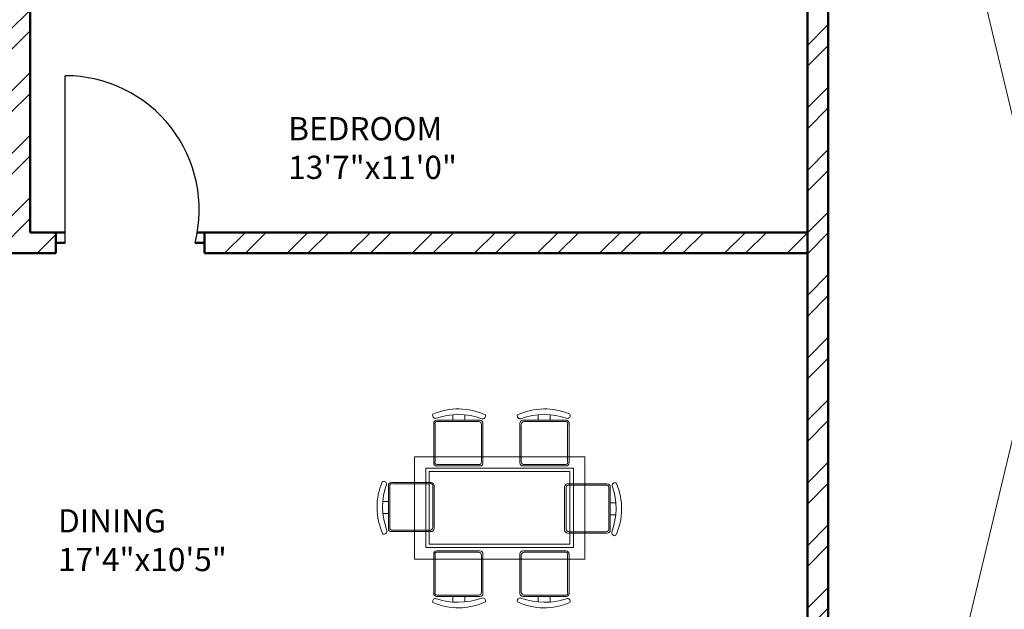
# Model space of a CAD drawing. Units: inches. Extents: x 1901 to 2863, y 888 to 2433.
# Tile 64 of 91: x 2169 to 2381, y 2002 to 2129. Entities that reach past the tile are written whole.
import ezdxf

# ---------------------------------------------------------------- set-up
doc = ezdxf.new("R2010")
doc.units = ezdxf.units.IN
for name, color, linetype, lineweight in [('A-ANNO-SYMB', 8, 'Continuous', 13), ('A-AREA-IDEN', 7, 'Continuous', 18), ('A-DOOR', 4, 'Continuous', 25), ('A-FURN', 8, 'Continuous', 18), ('A-WALL', 7, 'Continuous', 50), ('A-WALL-PATT', 8, 'Continuous', 13)]:
    doc.layers.add(name, color=color, linetype=linetype, lineweight=lineweight)
doc.styles.get("Standard").update_dxf_attribs({"font": 'arial.ttf'})

# ---------------------------------------------------------------- blocks, each defined once
blk = doc.blocks.new('DOOR-29')
blk.add_line((0, -0.02), (0, 35.98))
blk.add_arc((0, 7.12), 28.86, 345.6888, 90)

msp = doc.modelspace()

# ---------------------------------------------------------------- hatches: boundary and pattern name
at = {"layer": 'A-WALL-PATT'}
h = msp.add_hatch(dxfattribs=at)
h.set_pattern_fill('ANSI32', color=256)
h.paths.add_polyline_path([(2192.5, 2274.13), (2141.26, 2274.13), (2141.26, 2269.63), (2192.5, 2269.63)])
h.paths.add_polyline_path([(2259.93, 2274.13), (2216.5, 2274.13), (2216.5, 2269.63), (2255.43, 2269.63), (2255.43, 2214.63), (2250.81, 2214.63), (2250.81, 2210.13), (2259.93, 2210.13), (2259.93, 2215.13), (2271.76, 2215.13), (2271.76, 2217.38), (2271.76, 2219.63), (2259.93, 2219.63)])
h.paths.add_polyline_path([(2171.43, 2269.63), (2166.93, 2269.63), (2166.93, 2219.63), (2121.24, 2219.63), (2121.24, 2215.13), (2166.93, 2215.13), (2166.93, 2083.13), (2161.81, 2083.13), (2161.81, 2078.63), (2171.43, 2078.63), (2177, 2078.63), (2177, 2080.88), (2177, 2083.13), (2171.43, 2083.13), (2171.43, 2210.13), (2230.91, 2210.13), (2230.91, 2212.38), (2230.91, 2214.63), (2171.43, 2214.63)])
h.paths.add_polyline_path([(2117.26, 2274.13), (2089.43, 2274.13), (2089.43, 2219.63), (2081.14, 2219.63), (2081.14, 2215.13), (2089.43, 2215.13), (2098, 2215.13), (2098, 2217.38), (2098, 2219.63), (2093.93, 2219.63), (2093.93, 2269.63), (2117.26, 2269.63), (2117.26, 2271.88)])
h.paths.add_polyline_path([(2343.43, 2219.63), (2329.29, 2219.63), (2329.29, 2215.13), (2338.93, 2215.13), (2338.93, 2184.74), (2343.43, 2184.74)])
h.paths.add_polyline_path([(2338.93, 2083.13), (2329.29, 2083.13), (2208.97, 2083.13), (2208.97, 2078.63), (2338.93, 2078.63)])
h.paths.add_polyline_path([(2343.43, 2136.74), (2338.93, 2136.74), (2338.93, 1872.63), (2343.43, 1872.63)])
h.paths.add_polyline_path([(2343.43, 1863.63), (2397.68, 1863.63), (2397.68, 1821.63), (2384.14, 1821.63), (2384.14, 1812.63), (2418.33, 1812.63), (2418.33, 1817.13), (2418.33, 1821.63), (2406.68, 1821.63), (2406.68, 1863.63), (2459.5, 1863.63), (2459.5, 1821.63), (2447.14, 1821.63), (2447.14, 1812.63), (2459.5, 1812.63), (2468.5, 1812.63), (2468.5, 1872.63), (2394.43, 1872.63), (2334.43, 1872.63), (2334.43, 1812.63), (2343.43, 1812.63), (2353.25, 1812.63), (2353.25, 1821.63), (2343.43, 1821.63)])
h.paths.add_polyline_path([(2510.01, 1872.63), (2468.5, 1872.63), (2468.5, 1868.13), (2510.01, 1868.13)])
h.paths.add_polyline_path([(2514.01, 1817.13), (2468.5, 1817.13), (2468.5, 1812.63), (2482.11, 1812.63), (2482.11, 1800.61), (2486.61, 1800.61), (2486.61, 1812.63), (2514.01, 1812.63)])
h.paths.add_polyline_path([(2299.25, 1814.88), (2299.25, 1817.13), (2295.93, 1817.13), (2295.93, 1854.17), (2293.68, 1854.17), (2291.43, 1854.17), (2291.43, 1817.13), (2266.11, 1817.13), (2266.11, 1812.63), (2299.25, 1812.63)])
h.paths.add_polyline_path([(2218.11, 1817.13), (2206.46, 1817.13), (2171.43, 1817.13), (2171.43, 1949.13), (2190.1, 1949.13), (2190.1, 1953.63), (2163.47, 1953.63), (2163.47, 1949.13), (2166.93, 1949.13), (2166.93, 1817.13), (2114.3, 1817.13), (2114.3, 1812.63), (2218.11, 1812.63)])
h.paths.add_polyline_path([(2029.43, 1970.92), (2024.93, 1970.92), (2024.93, 1912.72), (2029.43, 1912.72)])
h.paths.add_polyline_path([(2132.3, 1953.63), (2113.93, 1953.63), (2113.93, 1975.89), (2111.68, 1975.89), (2109.43, 1975.89), (2109.43, 1953.63), (2029.43, 1953.63), (2029.43, 1949.13), (2132.3, 1949.13)])
h.paths.add_polyline_path([(2029.43, 1853.61), (2029.31, 1853.61), (2029.31, 1853.61), (2029.43, 1853.61), (2029.43, 1864.72), (2024.93, 1864.72), (2024.93, 1812.63), (2066.3, 1812.63), (2066.3, 1814.88), (2066.3, 1817.13), (2029.43, 1817.13)])
h.paths.add_polyline_path([(2122.93, 2010.09), (2120.68, 2010.09), (2118.43, 2010.09), (2118.43, 2006.13), (2029.43, 2006.13), (2029.43, 2001.63), (2109.43, 2001.63), (2109.43, 1998.04), (2113.93, 1998.04), (2113.93, 2001.63), (2122.93, 2001.63)])
h.paths.add_polyline_path([(2029.43, 2031.38), (2024.93, 2031.38), (2024.93, 1994.92), (2027.18, 1994.92), (2029.43, 1994.92)])
h.paths.add_polyline_path([(2029.43, 2136.74), (2024.93, 2136.74), (2024.93, 2067.38), (2027.18, 2067.38), (2029.43, 2067.38)])
h.paths.add_polyline_path([(2125.62, 2083.13), (2029.43, 2083.13), (2029.43, 2078.63), (2118.43, 2078.63), (2118.43, 2030.71), (2122.93, 2030.71), (2122.93, 2078.63), (2125.62, 2078.63)])
h.paths.add_polyline_path([(2029.43, 2215.13), (2040.47, 2215.13), (2040.47, 2217.38), (2040.47, 2219.63), (2024.93, 2219.63), (2024.93, 2184.74), (2029.43, 2184.74), (2029.43, 2187.78)])
h.paths.add_polyline_path([(2686.43, 2274.13), (2659.28, 2274.13), (2659.28, 2269.63), (2681.93, 2269.63), (2681.93, 2219.63), (2676.82, 2219.63), (2676.82, 2215.13), (2681.93, 2215.13), (2697.01, 2215.13), (2697.01, 2217.38), (2697.01, 2219.63), (2686.43, 2219.63)])
h.paths.add_polyline_path([(2609.93, 2269.63), (2635.28, 2269.63), (2635.28, 2274.13), (2571.43, 2274.13), (2571.43, 2269.63), (2605.43, 2269.63), (2605.43, 2214.63), (2549.1, 2214.63), (2549.1, 2210.13), (2605.43, 2210.13), (2605.43, 2083.13), (2601.01, 2083.13), (2601.01, 2080.88), (2601.01, 2078.63), (2609.93, 2078.63), (2616.16, 2078.63), (2616.16, 2080.88), (2616.16, 2083.13), (2609.93, 2083.13), (2609.93, 2215.13), (2651.46, 2215.13), (2651.46, 2217.38), (2651.46, 2219.63), (2609.93, 2219.63)])
h.paths.add_polyline_path([(2521.43, 2269.63), (2547.43, 2269.63), (2547.43, 2271.88), (2547.43, 2274.13), (2516.93, 2274.13), (2516.93, 2219.63), (2506.41, 2219.63), (2506.41, 2215.13), (2516.93, 2215.13), (2516.93, 2210.13), (2525.4, 2210.13), (2525.4, 2212.38), (2525.4, 2214.63), (2521.43, 2214.63)])
h.paths.add_polyline_path([(2456.01, 2219.63), (2439.43, 2219.63), (2439.43, 2187.89), (2443.93, 2187.89), (2443.93, 2215.13), (2456.01, 2215.13)])
h.paths.add_polyline_path([(2752.93, 2219.63), (2739.48, 2219.63), (2739.48, 2215.13), (2748.43, 2215.13), (2748.43, 2187.89), (2752.93, 2187.89)])
h.paths.add_polyline_path([(2752.93, 2139.89), (2748.43, 2139.89), (2748.43, 2083.13), (2648.42, 2083.13), (2648.42, 2078.63), (2654.93, 2078.63), (2654.93, 2039.44), (2659.43, 2039.44), (2659.43, 2078.63), (2748.43, 2078.63), (2748.43, 2063.43), (2752.93, 2063.43)])
h.paths.add_polyline_path([(2752.93, 2010.63), (2659.43, 2010.63), (2659.43, 2015.65), (2654.93, 2015.65), (2654.93, 2010.63), (2605.43, 2010.63), (2605.43, 1920.97), (2609.93, 1920.97), (2609.93, 2006.13), (2748.43, 2006.13), (2748.43, 1982.47), (2752.93, 1982.47)])
h.paths.add_polyline_path([(2752.93, 2027.43), (2748.43, 2027.43), (2748.43, 2010.63), (2752.93, 2010.63)])
h.paths.add_polyline_path([(2748.43, 1886.13), (2609.93, 1886.13), (2609.93, 1889.72), (2605.43, 1889.72), (2605.43, 1861.26), (2609.93, 1861.26), (2609.93, 1881.63), (2748.43, 1881.63)])
h.paths.add_polyline_path([(2456.86, 2228.83), (2498.4, 2228.83), (2498.4, 2247.49), (2456.86, 2247.49)], flags=9)
h.paths.add_polyline_path([(2038.6, 2237.42), (2080.17, 2237.42), (2080.17, 2256.08), (2038.6, 2256.08)], flags=9)
h.paths.add_polyline_path([(2292.01, 1062.39), (2539.93, 1062.39), (2539.93, 1099.49), (2292.01, 1099.49)], flags=9)
h.paths.add_polyline_path([(2424.91, 1832.25), (2448.51, 1832.25), (2448.51, 1846.68), (2424.91, 1846.68)], flags=25)
h.paths.add_polyline_path([(2359.08, 1832.25), (2382.68, 1832.25), (2382.68, 1846.68), (2359.08, 1846.68)], flags=25)
h.paths.add_polyline_path([(2352.9, 1684.8), (2367.54, 1684.8), (2367.54, 1697.17), (2352.9, 1697.17)], flags=9)
h.paths.add_polyline_path([(2079.29, 1755.83), (2169.02, 1755.83), (2169.02, 1774.37), (2079.29, 1774.37)], flags=9)
h.paths.add_polyline_path([(2404.09, 1373.86), (2404.09, 1463.59), (2385.54, 1463.59), (2385.54, 1373.86)], flags=9)
h.paths.add_polyline_path([(2268.09, 2236.37), (2309.64, 2236.37), (2309.64, 2255.03), (2268.09, 2255.03)], flags=9)
h.paths.add_polyline_path([(2575.96, 1700.95), (2665.7, 1700.95), (2665.7, 1719.5), (2575.96, 1719.5)], flags=9)
h.paths.add_polyline_path([(2302.96, 1878.47), (2329.52, 1878.47), (2329.52, 1888.78), (2302.96, 1888.78)], flags=9)
h.paths.add_polyline_path([(2097.42, 2240.58), (2126.57, 2240.58), (2126.57, 2259.23), (2097.42, 2259.23)], flags=9)
h.paths.add_polyline_path([(2208.72, 2246.12), (2237.88, 2246.12), (2237.88, 2264.78), (2208.72, 2264.78)], flags=9)
h.paths.add_polyline_path([(2038.15, 1925.96), (2076.99, 1925.96), (2076.99, 1944.62), (2038.15, 1944.62)], flags=9)
h.paths.add_polyline_path([(2239.14, 1926.67), (2288.46, 1926.67), (2288.46, 1945.33), (2239.14, 1945.33)], flags=9)
h.paths.add_polyline_path([(2175.43, 2007.33), (2212.36, 2007.33), (2212.36, 2025.99), (2175.43, 2025.99)], flags=9)
h.paths.add_polyline_path([(2225.03, 2091.79), (2263.87, 2091.79), (2263.87, 2110.45), (2225.03, 2110.45)], flags=9)
h.paths.add_polyline_path([(2035.4, 2098.48), (2074.24, 2098.48), (2074.24, 2117.14), (2035.4, 2117.14)], flags=9)
h.paths.add_polyline_path([(2050.1, 2029.21), (2083.26, 2029.21), (2083.26, 2047.87), (2050.1, 2047.87)], flags=9)
h.paths.add_polyline_path([(2069.68, 1956.72), (2098.83, 1956.72), (2098.83, 1975.38), (2069.68, 1975.38)], flags=25)
h.paths.add_polyline_path([(2328.62, 1753.34), (2361.66, 1753.34), (2361.66, 1771.99), (2328.62, 1771.99)], flags=9)
h.paths.add_polyline_path([(2395.16, 2060.89), (2395.16, 2140.65), (2378.68, 2140.65), (2378.68, 2060.89)], flags=9)
h.paths.add_polyline_path([(2463.73, 2059.02), (2492.89, 2059.02), (2492.89, 2077.68), (2463.73, 2077.68)], flags=9)
h.paths.add_polyline_path([(2458.03, 2181.54), (2496.87, 2181.54), (2496.87, 2200.19), (2458.03, 2200.19)], flags=9)
h.paths.add_polyline_path([(2527.58, 2243.07), (2556.73, 2243.07), (2556.73, 2261.73), (2527.58, 2261.73)], flags=9)
h.paths.add_polyline_path([(2694.46, 2232.77), (2736.03, 2232.77), (2736.03, 2251.42), (2694.46, 2251.42)], flags=9)
h.paths.add_polyline_path([(2637.82, 2249.22), (2666.98, 2249.22), (2666.98, 2267.88), (2637.82, 2267.88)], flags=9)
h.paths.add_polyline_path([(2623.69, 2183.54), (2662.53, 2183.54), (2662.53, 2202.2), (2623.69, 2202.2)], flags=9)
h.paths.add_polyline_path([(2691.97, 2021.5), (2725.12, 2021.5), (2725.12, 2040.16), (2691.97, 2040.16)], flags=9)
h.paths.add_polyline_path([(2621.04, 1975.91), (2662.34, 1975.91), (2662.34, 1994.57), (2621.04, 1994.57)], flags=25)
h.paths.add_polyline_path([(2479.03, 1927.62), (2519.84, 1927.62), (2519.84, 1946.28), (2479.03, 1946.28)], flags=9)
h.paths.add_polyline_path([(2670.94, 1849.08), (2716.01, 1849.08), (2716.01, 1867.73), (2670.94, 1867.73)], flags=9)
h.paths.add_polyline_path([(2523.61, 1782.96), (2550.17, 1782.96), (2550.17, 1793.26), (2523.61, 1793.26)], flags=9)
h.paths.add_polyline_path([(2450.84, 1207.33), (2492.39, 1207.33), (2492.39, 1225.99), (2450.84, 1225.99)], flags=9)
h.paths.add_polyline_path([(2527.75, 1203.84), (2556.91, 1203.84), (2556.91, 1222.5), (2527.75, 1222.5)], flags=9)
h.paths.add_polyline_path([(2639.11, 1207.2), (2668.27, 1207.2), (2668.27, 1225.86), (2639.11, 1225.86)], flags=9)
h.paths.add_polyline_path([(2692.59, 1218.97), (2734.17, 1218.97), (2734.17, 1237.62), (2692.59, 1237.62)], flags=9)
h.paths.add_polyline_path([(2669.27, 1366.33), (2708.11, 1366.33), (2708.11, 1384.99), (2669.27, 1384.99)], flags=9)
h.paths.add_polyline_path([(2463.31, 1358.03), (2502.15, 1358.03), (2502.15, 1376.69), (2463.31, 1376.69)], flags=9)
h.paths.add_polyline_path([(2494.72, 1449.96), (2531.65, 1449.96), (2531.65, 1468.62), (2494.72, 1468.62)], flags=9)
h.paths.add_polyline_path([(2675.57, 1422.16), (2708.72, 1422.16), (2708.72, 1440.81), (2675.57, 1440.81)], flags=9)
h.paths.add_polyline_path([(2685.63, 1493.89), (2714.79, 1493.89), (2714.79, 1512.55), (2685.63, 1512.55)], flags=9)
h.paths.add_polyline_path([(2686.8, 1529.91), (2725.65, 1529.91), (2725.65, 1548.57), (2686.8, 1548.57)], flags=9)
h.paths.add_polyline_path([(2503.65, 1537.99), (2552.97, 1537.99), (2552.97, 1556.65), (2503.65, 1556.65)], flags=9)
h.paths.add_polyline_path([(2291.71, 1643.5), (2318.28, 1643.5), (2318.28, 1653.81), (2291.71, 1653.81)], flags=9)
h.paths.add_polyline_path([(2450.63, 1610.52), (2477.19, 1610.52), (2477.19, 1620.82), (2450.63, 1620.82)], flags=9)
h.paths.add_polyline_path([(2359.99, 1551.81), (2422.25, 1551.81), (2422.25, 1562.12), (2359.99, 1562.12)], flags=9)
h.paths.add_polyline_path([(2280.11, 1249.01), (2321.65, 1249.01), (2321.65, 1267.66), (2280.11, 1267.66)], flags=9)
h.paths.add_polyline_path([(2164.06, 1274.23), (2193.22, 1274.23), (2193.22, 1292.89), (2164.06, 1292.89)], flags=9)
h.paths.add_polyline_path([(2118.21, 1277.69), (2151.25, 1277.69), (2151.25, 1296.35), (2118.21, 1296.35)], flags=9)
h.paths.add_polyline_path([(2031.95, 1268.53), (2073.52, 1268.53), (2073.52, 1287.19), (2031.95, 1287.19)], flags=9)
h.paths.add_polyline_path([(2050.2, 1409.08), (2089.04, 1409.08), (2089.04, 1427.74), (2050.2, 1427.74)], flags=9)
h.paths.add_polyline_path([(2243.74, 1421.03), (2282.58, 1421.03), (2282.58, 1439.69), (2243.74, 1439.69)], flags=9)
h.paths.add_polyline_path([(2190.75, 1509.77), (2231.56, 1509.77), (2231.56, 1528.43), (2190.75, 1528.43)], flags=9)
h.paths.add_polyline_path([(2058.39, 1475.42), (2091.55, 1475.42), (2091.55, 1494.07), (2058.39, 1494.07)], flags=9)
h.paths.add_polyline_path([(2062.45, 1553.09), (2091.6, 1553.09), (2091.6, 1571.75), (2062.45, 1571.75)], flags=9)
h.paths.add_polyline_path([(2219.52, 1590.37), (2266.15, 1590.37), (2266.15, 1609.02), (2219.52, 1609.02)], flags=9)
h.paths.add_polyline_path([(2041.07, 1584.19), (2079.91, 1584.19), (2079.91, 1602.85), (2041.07, 1602.85)], flags=9)
h = msp.add_hatch(dxfattribs=at)
h.set_pattern_fill('ANSI32', color=256)
h.paths.add_polyline_path([(2443.93, 2139.89), (2439.43, 2139.89), (2439.43, 2069.35), (2441.68, 2069.35), (2443.93, 2069.35), (2443.93, 2078.63), (2521.93, 2078.63), (2521.93, 2075.07), (2524.18, 2075.07), (2526.43, 2075.07), (2526.43, 2078.63), (2571.75, 2078.63), (2571.75, 2080.88), (2571.75, 2083.13), (2443.93, 2083.13)])
h.paths.add_polyline_path([(2526.43, 2054.63), (2524.18, 2054.63), (2521.93, 2054.63), (2521.93, 2030.63), (2443.93, 2030.63), (2443.93, 2045.35), (2439.43, 2045.35), (2439.43, 1983.87), (2443.93, 1983.87), (2443.93, 2026.13), (2521.93, 2026.13), (2526.43, 2026.13)])
h.paths.add_polyline_path([(2443.93, 1923.87), (2439.43, 1923.87), (2439.43, 1872.63), (2443.93, 1872.63)])
h.paths.add_polyline_path([(2636.23, 1766.13), (2609.93, 1766.13), (2609.93, 1779.79), (2605.43, 1779.79), (2605.43, 1766.13), (2486.61, 1766.13), (2486.61, 1770.67), (2482.11, 1770.67), (2482.11, 1766.13), (2482.11, 1761.63), (2636.23, 1761.63), (2636.23, 1763.88)])
h.paths.add_polyline_path([(2519.54, 1663.38), (2519.54, 1665.63), (2494.93, 1665.63), (2481.83, 1665.63), (2481.83, 1663.38), (2481.83, 1661.13), (2490.43, 1661.13), (2490.43, 1640.16), (2494.93, 1640.16), (2494.93, 1661.13), (2519.54, 1661.13)])
h.paths.add_polyline_path([(2443.93, 1712.13), (2443.93, 1716.63), (2414.46, 1716.63), (2414.46, 1712.13), (2439.43, 1712.13), (2439.43, 1545.51), (2443.93, 1545.51), (2443.93, 1661.13), (2448.47, 1661.13), (2448.47, 1665.63), (2443.93, 1665.63)])
h.paths.add_polyline_path([(2343.43, 1712.13), (2365.52, 1712.13), (2365.52, 1714.38), (2365.52, 1716.63), (2333.87, 1716.63), (2333.87, 1714.38), (2333.87, 1712.13), (2338.93, 1712.13), (2338.93, 1575.63), (2338.93, 1545.51), (2343.43, 1545.51), (2343.43, 1547.51), (2343.43, 1580.13)])
h.paths.add_polyline_path([(2752.93, 1665.63), (2579.54, 1665.63), (2579.54, 1661.13), (2615.93, 1661.13), (2615.93, 1529.13), (2598.93, 1529.13), (2598.93, 1524.63), (2623.13, 1524.63), (2623.13, 1526.88), (2623.13, 1529.13), (2620.43, 1529.13), (2620.43, 1661.13), (2748.43, 1661.13), (2748.43, 1633.5), (2752.93, 1633.5)])
h.paths.add_polyline_path([(2752.93, 1419.93), (2748.43, 1419.93), (2748.43, 1400.13), (2659.43, 1400.13), (2659.43, 1444.33), (2657.18, 1444.33), (2654.93, 1444.33), (2654.93, 1400.13), (2643.65, 1400.13), (2643.65, 1395.63), (2748.43, 1395.63), (2748.43, 1364.04), (2752.93, 1364.04)])
h.paths.add_polyline_path([(2752.93, 1492.88), (2748.43, 1492.88), (2748.43, 1476.63), (2667.43, 1476.63), (2667.43, 1479.71), (2665.18, 1479.71), (2662.93, 1479.71), (2662.93, 1476.63), (2654.93, 1476.63), (2654.93, 1469.54), (2659.43, 1469.54), (2659.43, 1472.13), (2748.43, 1472.13), (2748.43, 1455.93), (2752.93, 1455.93)])
h.paths.add_polyline_path([(2752.93, 1304.04), (2748.43, 1304.04), (2748.43, 1263.63), (2738.66, 1263.63), (2738.66, 1259.13), (2752.93, 1259.13)])
h.paths.add_polyline_path([(2685.93, 1259.13), (2695.49, 1259.13), (2695.49, 1261.38), (2695.49, 1263.63), (2677.84, 1263.63), (2677.84, 1261.38), (2677.84, 1259.13), (2681.43, 1259.13), (2681.43, 1203.63), (2653.28, 1203.63), (2653.28, 1199.13), (2685.93, 1199.13), (2685.93, 1203.63)])
h.paths.add_polyline_path([(2609.43, 1395.63), (2611.85, 1395.63), (2611.85, 1400.13), (2598.89, 1400.13), (2598.89, 1397.88), (2598.89, 1395.63), (2604.93, 1395.63), (2604.93, 1268.13), (2554.73, 1268.13), (2554.73, 1265.88), (2554.73, 1263.63), (2604.93, 1263.63), (2604.93, 1203.63), (2571.31, 1203.63), (2571.31, 1199.13), (2604.93, 1199.13), (2629.28, 1199.13), (2629.28, 1201.38), (2629.28, 1203.63), (2609.43, 1203.63), (2609.43, 1258.63), (2609.43, 1259.13), (2654.8, 1259.13), (2654.8, 1263.63), (2609.43, 1263.63)])
h.paths.add_polyline_path([(2443.93, 1304.04), (2439.43, 1304.04), (2439.43, 1259.13), (2443.93, 1259.13), (2456.16, 1259.13), (2456.16, 1261.38), (2456.16, 1263.63), (2443.93, 1263.63)])
h.paths.add_polyline_path([(2525.43, 1263.63), (2531.78, 1263.63), (2531.78, 1268.13), (2520.93, 1268.13), (2520.93, 1263.63), (2511.41, 1263.63), (2511.41, 1259.13), (2520.93, 1259.13), (2520.93, 1199.13), (2547.31, 1199.13), (2547.31, 1201.38), (2547.31, 1203.63), (2525.43, 1203.63)])
h.paths.add_polyline_path([(2443.93, 1434.84), (2439.43, 1434.84), (2439.43, 1364.04), (2441.68, 1364.04), (2443.93, 1364.04)])
h.paths.add_polyline_path([(2567.13, 1400.13), (2443.93, 1400.13), (2443.93, 1395.63), (2567.13, 1395.63)])
h.paths.add_polyline_path([(2443.93, 1545.51), (2439.43, 1545.51), (2439.43, 1494.84), (2443.93, 1494.84)])
h.paths.add_polyline_path([(2494.93, 1553.35), (2492.68, 1553.35), (2490.43, 1553.35), (2490.43, 1524.63), (2494.93, 1524.63), (2525.94, 1524.63), (2525.94, 1526.88), (2525.94, 1529.13), (2494.93, 1529.13)])
h.paths.add_polyline_path([(2752.93, 1573.5), (2748.43, 1573.5), (2748.43, 1529.13), (2657.76, 1529.13), (2657.76, 1524.63), (2662.93, 1524.63), (2662.93, 1498.63), (2667.43, 1498.63), (2667.43, 1524.63), (2748.43, 1524.63), (2748.43, 1516.88), (2752.93, 1516.88)])
h.paths.add_polyline_path([(2038.6, 2237.42), (2080.17, 2237.42), (2080.17, 2256.08), (2038.6, 2256.08)], flags=9)
h.paths.add_polyline_path([(2292.01, 1062.39), (2539.93, 1062.39), (2539.93, 1099.49), (2292.01, 1099.49)], flags=9)
h.paths.add_polyline_path([(2424.91, 1832.25), (2448.51, 1832.25), (2448.51, 1846.68), (2424.91, 1846.68)], flags=9)
h.paths.add_polyline_path([(2359.08, 1832.25), (2382.68, 1832.25), (2382.68, 1846.68), (2359.08, 1846.68)], flags=9)
h.paths.add_polyline_path([(2352.9, 1684.8), (2367.54, 1684.8), (2367.54, 1697.17), (2352.9, 1697.17)], flags=9)
h.paths.add_polyline_path([(2079.29, 1755.83), (2169.02, 1755.83), (2169.02, 1774.37), (2079.29, 1774.37)], flags=9)
h.paths.add_polyline_path([(2404.09, 1373.86), (2404.09, 1463.59), (2385.54, 1463.59), (2385.54, 1373.86)], flags=9)
h.paths.add_polyline_path([(2268.09, 2236.37), (2309.64, 2236.37), (2309.64, 2255.03), (2268.09, 2255.03)], flags=9)
h.paths.add_polyline_path([(2575.96, 1700.95), (2665.7, 1700.95), (2665.7, 1719.5), (2575.96, 1719.5)], flags=9)
h.paths.add_polyline_path([(2302.96, 1878.47), (2329.52, 1878.47), (2329.52, 1888.78), (2302.96, 1888.78)], flags=9)
h.paths.add_polyline_path([(2097.42, 2240.58), (2126.57, 2240.58), (2126.57, 2259.23), (2097.42, 2259.23)], flags=9)
h.paths.add_polyline_path([(2208.72, 2246.12), (2237.88, 2246.12), (2237.88, 2264.78), (2208.72, 2264.78)], flags=9)
h.paths.add_polyline_path([(2038.15, 1925.96), (2076.99, 1925.96), (2076.99, 1944.62), (2038.15, 1944.62)], flags=9)
h.paths.add_polyline_path([(2239.14, 1926.67), (2288.46, 1926.67), (2288.46, 1945.33), (2239.14, 1945.33)], flags=9)
h.paths.add_polyline_path([(2175.43, 2007.33), (2212.36, 2007.33), (2212.36, 2025.99), (2175.43, 2025.99)], flags=9)
h.paths.add_polyline_path([(2225.03, 2091.79), (2263.87, 2091.79), (2263.87, 2110.45), (2225.03, 2110.45)], flags=9)
h.paths.add_polyline_path([(2035.4, 2098.48), (2074.24, 2098.48), (2074.24, 2117.14), (2035.4, 2117.14)], flags=9)
h.paths.add_polyline_path([(2050.1, 2029.21), (2083.26, 2029.21), (2083.26, 2047.87), (2050.1, 2047.87)], flags=9)
h.paths.add_polyline_path([(2069.68, 1956.72), (2098.83, 1956.72), (2098.83, 1975.38), (2069.68, 1975.38)], flags=9)
h.paths.add_polyline_path([(2328.62, 1753.34), (2361.66, 1753.34), (2361.66, 1771.99), (2328.62, 1771.99)], flags=9)
h.paths.add_polyline_path([(2395.16, 2060.89), (2395.16, 2140.65), (2378.68, 2140.65), (2378.68, 2060.89)], flags=9)
h.paths.add_polyline_path([(2463.73, 2059.02), (2492.89, 2059.02), (2492.89, 2077.68), (2463.73, 2077.68)], flags=9)
h.paths.add_polyline_path([(2458.03, 2181.54), (2496.87, 2181.54), (2496.87, 2200.19), (2458.03, 2200.19)], flags=9)
h.paths.add_polyline_path([(2456.86, 2228.83), (2498.4, 2228.83), (2498.4, 2247.49), (2456.86, 2247.49)], flags=9)
h.paths.add_polyline_path([(2527.58, 2243.07), (2556.73, 2243.07), (2556.73, 2261.73), (2527.58, 2261.73)], flags=9)
h.paths.add_polyline_path([(2694.46, 2232.77), (2736.03, 2232.77), (2736.03, 2251.42), (2694.46, 2251.42)], flags=9)
h.paths.add_polyline_path([(2637.82, 2249.22), (2666.98, 2249.22), (2666.98, 2267.88), (2637.82, 2267.88)], flags=9)
h.paths.add_polyline_path([(2623.69, 2183.54), (2662.53, 2183.54), (2662.53, 2202.2), (2623.69, 2202.2)], flags=9)
h.paths.add_polyline_path([(2691.97, 2021.5), (2725.12, 2021.5), (2725.12, 2040.16), (2691.97, 2040.16)], flags=9)
h.paths.add_polyline_path([(2621.04, 1975.91), (2662.34, 1975.91), (2662.34, 1994.57), (2621.04, 1994.57)], flags=9)
h.paths.add_polyline_path([(2479.03, 1927.62), (2519.84, 1927.62), (2519.84, 1946.28), (2479.03, 1946.28)], flags=9)
h.paths.add_polyline_path([(2670.94, 1849.08), (2716.01, 1849.08), (2716.01, 1867.73), (2670.94, 1867.73)], flags=9)
h.paths.add_polyline_path([(2523.61, 1782.96), (2550.17, 1782.96), (2550.17, 1793.26), (2523.61, 1793.26)], flags=9)
h.paths.add_polyline_path([(2450.84, 1207.33), (2492.39, 1207.33), (2492.39, 1225.99), (2450.84, 1225.99)], flags=9)
h.paths.add_polyline_path([(2527.75, 1203.84), (2556.91, 1203.84), (2556.91, 1222.5), (2527.75, 1222.5)], flags=9)
h.paths.add_polyline_path([(2639.11, 1207.2), (2668.27, 1207.2), (2668.27, 1225.86), (2639.11, 1225.86)], flags=9)
h.paths.add_polyline_path([(2692.59, 1218.97), (2734.17, 1218.97), (2734.17, 1237.62), (2692.59, 1237.62)], flags=9)
h.paths.add_polyline_path([(2669.27, 1366.33), (2708.11, 1366.33), (2708.11, 1384.99), (2669.27, 1384.99)], flags=25)
h.paths.add_polyline_path([(2463.31, 1358.03), (2502.15, 1358.03), (2502.15, 1376.69), (2463.31, 1376.69)], flags=9)
h.paths.add_polyline_path([(2494.72, 1449.96), (2531.65, 1449.96), (2531.65, 1468.62), (2494.72, 1468.62)], flags=9)
h.paths.add_polyline_path([(2675.57, 1422.16), (2708.72, 1422.16), (2708.72, 1440.81), (2675.57, 1440.81)], flags=25)
h.paths.add_polyline_path([(2685.63, 1493.89), (2714.79, 1493.89), (2714.79, 1512.55), (2685.63, 1512.55)], flags=9)
h.paths.add_polyline_path([(2686.8, 1529.91), (2725.65, 1529.91), (2725.65, 1548.57), (2686.8, 1548.57)], flags=25)
h.paths.add_polyline_path([(2503.65, 1537.99), (2552.97, 1537.99), (2552.97, 1556.65), (2503.65, 1556.65)], flags=9)
h.paths.add_polyline_path([(2291.71, 1643.5), (2318.28, 1643.5), (2318.28, 1653.81), (2291.71, 1653.81)], flags=9)
h.paths.add_polyline_path([(2450.63, 1610.52), (2477.19, 1610.52), (2477.19, 1620.82), (2450.63, 1620.82)], flags=9)
h.paths.add_polyline_path([(2359.99, 1551.81), (2422.25, 1551.81), (2422.25, 1562.12), (2359.99, 1562.12)], flags=9)
h.paths.add_polyline_path([(2280.11, 1249.01), (2321.65, 1249.01), (2321.65, 1267.66), (2280.11, 1267.66)], flags=9)
h.paths.add_polyline_path([(2164.06, 1274.23), (2193.22, 1274.23), (2193.22, 1292.89), (2164.06, 1292.89)], flags=9)
h.paths.add_polyline_path([(2118.21, 1277.69), (2151.25, 1277.69), (2151.25, 1296.35), (2118.21, 1296.35)], flags=9)
h.paths.add_polyline_path([(2031.95, 1268.53), (2073.52, 1268.53), (2073.52, 1287.19), (2031.95, 1287.19)], flags=9)
h.paths.add_polyline_path([(2050.2, 1409.08), (2089.04, 1409.08), (2089.04, 1427.74), (2050.2, 1427.74)], flags=9)
h.paths.add_polyline_path([(2243.74, 1421.03), (2282.58, 1421.03), (2282.58, 1439.69), (2243.74, 1439.69)], flags=9)
h.paths.add_polyline_path([(2190.75, 1509.77), (2231.56, 1509.77), (2231.56, 1528.43), (2190.75, 1528.43)], flags=9)
h.paths.add_polyline_path([(2058.39, 1475.42), (2091.55, 1475.42), (2091.55, 1494.07), (2058.39, 1494.07)], flags=9)
h.paths.add_polyline_path([(2062.45, 1553.09), (2091.6, 1553.09), (2091.6, 1571.75), (2062.45, 1571.75)], flags=9)
h.paths.add_polyline_path([(2219.52, 1590.37), (2266.15, 1590.37), (2266.15, 1609.02), (2219.52, 1609.02)], flags=9)
h.paths.add_polyline_path([(2041.07, 1584.19), (2079.91, 1584.19), (2079.91, 1602.85), (2041.07, 1602.85)], flags=9)

# ---------------------------------------------------------------- linework, layer by layer
at = {"layer": 'A-ANNO-SYMB'}
for p, q in [((2343.43, 2274.13), (2439.43, 1872.63)), ((2343.43, 1872.63), (2439.43, 2274.13))]:
    msp.add_line(p, q, dxfattribs=at)
at = {"layer": 'A-FURN'}
for points in [[(2258.77, 2043.05, -0.175809), (2268.77, 2042.98, 0.578392), (2269.53, 2043.81, 0.214524), (2258.24, 2043.96, 0.552014), (2258.77, 2043.05, -0.065079)], [(2258.77, 2043.05, -0.175809), (2268.77, 2042.98, 0.578392), (2269.53, 2043.81, 0.214524), (2258.24, 2043.96, 0.552014), (2258.77, 2043.05, -0.065079)], [(2265.09, 2042.65), (2265.09, 2043.83, -0.064759)], [(2265.09, 2042.65), (2265.09, 2043.83, -0.064759)], [(2277.2, 2042.98, -0.578392), (2276.44, 2043.81, -0.214524), (2287.73, 2043.96, -0.552014), (2287.2, 2043.05, 0.175809), (2277.2, 2042.98)], [(2277.2, 2042.98, -0.578392), (2276.44, 2043.81, -0.214524), (2287.73, 2043.96, -0.552014), (2287.2, 2043.05, 0.175809), (2277.2, 2042.98)], [(2280.88, 2042.65), (2280.88, 2043.83, 0.064759)], [(2280.88, 2042.65), (2280.88, 2043.83, 0.064759)], [(2268.35, 2042.65), (2259.06, 2042.65, 0.414214), (2258.41, 2042), (2258.41, 2033.46, 0.414214), (2259.06, 2032.81), (2268.35, 2032.81, 0.414214), (2269, 2033.46), (2269, 2042, 0.414214), (2268.35, 2042.65)], [(2268.35, 2042.65), (2259.06, 2042.65, 0.414214), (2258.41, 2042), (2258.41, 2033.46, 0.414214), (2259.06, 2032.81), (2268.35, 2032.81, 0.414214), (2269, 2033.46), (2269, 2042, 0.414214), (2268.35, 2042.65)], [(2286.91, 2042.65, -0.414214), (2287.56, 2042), (2287.56, 2033.46, -0.414214), (2286.91, 2032.81), (2277.62, 2032.81, -0.414214), (2276.97, 2033.46), (2276.97, 2042, -0.414214), (2277.62, 2042.65), (2286.91, 2042.65)], [(2286.91, 2042.65, -0.414214), (2287.56, 2042), (2287.56, 2033.46, -0.414214), (2286.91, 2032.81), (2277.62, 2032.81, -0.414214), (2276.97, 2033.46), (2276.97, 2042, -0.414214), (2277.62, 2042.65), (2286.91, 2042.65)], [(2248.3, 2018.9, -0.578392), (2247.47, 2018.14, -0.214524), (2247.32, 2029.43, -0.552014), (2248.23, 2028.9, 0.175809), (2248.3, 2018.9)], [(2248.3, 2018.9, -0.578392), (2247.47, 2018.14, -0.214524), (2247.32, 2029.43, -0.552014), (2248.23, 2028.9, 0.175809), (2248.3, 2018.9)], [(2248.63, 2028.61, -0.414214), (2249.28, 2029.26), (2257.82, 2029.26, -0.414214), (2258.47, 2028.61), (2258.47, 2019.32, -0.414214), (2257.82, 2018.67), (2249.28, 2018.67, -0.414214), (2248.63, 2019.32), (2248.63, 2028.61)], [(2248.63, 2028.61, -0.414214), (2249.28, 2029.26), (2257.82, 2029.26, -0.414214), (2258.47, 2028.61), (2258.47, 2019.32, -0.414214), (2257.82, 2018.67), (2249.28, 2018.67, -0.414214), (2248.63, 2019.32), (2248.63, 2028.61)], [(2296.45, 2028.29, 0.414214), (2295.8, 2028.94), (2287.26, 2028.94, 0.414214), (2286.61, 2028.29), (2286.61, 2019, 0.414214), (2287.26, 2018.35), (2295.8, 2018.35, 0.414214), (2296.45, 2019), (2296.45, 2028.29)], [(2296.45, 2028.29, 0.414214), (2295.8, 2028.94), (2287.26, 2028.94, 0.414214), (2286.61, 2028.29), (2286.61, 2019, 0.414214), (2287.26, 2018.35), (2295.8, 2018.35, 0.414214), (2296.45, 2019), (2296.45, 2028.29)], [(2296.85, 2028.58, -0.175809), (2296.78, 2018.58, 0.578392), (2297.61, 2017.82, 0.214524), (2297.76, 2029.11, 0.552014), (2296.85, 2028.58, -0.065079)], [(2296.85, 2028.58, -0.175809), (2296.78, 2018.58, 0.578392), (2297.61, 2017.82, 0.214524), (2297.76, 2029.11, 0.552014), (2296.85, 2028.58, -0.065079)], [(2248.63, 2022.58), (2247.46, 2022.58, 0.064759)], [(2248.63, 2022.58), (2247.46, 2022.58, 0.064759)], [(2296.45, 2022.27), (2297.63, 2022.27, -0.064759)], [(2296.45, 2022.27), (2297.63, 2022.27, -0.064759)], [(2268.35, 2004.69), (2259.06, 2004.69, -0.414214), (2258.41, 2005.34), (2258.41, 2013.88, -0.414214), (2259.06, 2014.53), (2268.35, 2014.53, -0.414214), (2269, 2013.88), (2269, 2005.34, -0.414214), (2268.35, 2004.69)], [(2268.35, 2004.69), (2259.06, 2004.69, -0.414214), (2258.41, 2005.34), (2258.41, 2013.88, -0.414214), (2259.06, 2014.53), (2268.35, 2014.53, -0.414214), (2269, 2013.88), (2269, 2005.34, -0.414214), (2268.35, 2004.69)], [(2286.91, 2004.69, 0.414214), (2287.56, 2005.34), (2287.56, 2013.88, 0.414214), (2286.91, 2014.53), (2277.62, 2014.53, 0.414214), (2276.97, 2013.88), (2276.97, 2005.34, 0.414214), (2277.62, 2004.69), (2286.91, 2004.69)], [(2286.91, 2004.69, 0.414214), (2287.56, 2005.34), (2287.56, 2013.88, 0.414214), (2286.91, 2014.53), (2277.62, 2014.53, 0.414214), (2276.97, 2013.88), (2276.97, 2005.34, 0.414214), (2277.62, 2004.69), (2286.91, 2004.69)], [(2268.77, 2004.37, -0.578392), (2269.53, 2003.54, -0.214524), (2258.24, 2003.38, -0.552014), (2258.77, 2004.29, 0.175809), (2268.77, 2004.37)], [(2268.77, 2004.37, -0.578392), (2269.53, 2003.53, -0.214524), (2258.24, 2003.38, -0.552014), (2258.77, 2004.29, 0.175809), (2268.77, 2004.37)], [(2265.09, 2004.69), (2265.09, 2003.52, 0.064759)], [(2265.09, 2004.69), (2265.09, 2003.52, 0.064759)], [(2287.2, 2004.29, -0.175809), (2277.2, 2004.37, 0.578392), (2276.44, 2003.54, 0.214524), (2287.73, 2003.38, 0.552014), (2287.2, 2004.29, -0.065079)], [(2287.2, 2004.29, -0.175809), (2277.2, 2004.37, 0.578392), (2276.44, 2003.53, 0.214524), (2287.73, 2003.38, 0.552014), (2287.2, 2004.29, -0.065079)], [(2280.88, 2004.69), (2280.88, 2003.52, -0.064759)], [(2280.88, 2004.69), (2280.88, 2003.52, -0.064759)]]:
    msp.add_lwpolyline(points, format="xyb", dxfattribs=at)
for points in [[(2262.49, 2043.85), (2262.49, 2042.65)], [(2262.49, 2043.85), (2262.49, 2042.65)], [(2283.48, 2043.85), (2283.48, 2042.65)], [(2283.48, 2043.85), (2283.48, 2042.65)], [(2247.43, 2025.18), (2248.63, 2025.18)], [(2247.43, 2025.18), (2248.63, 2025.18)], [(2297.65, 2024.87), (2296.45, 2024.87)], [(2297.65, 2024.87), (2296.45, 2024.87)], [(2262.49, 2003.5), (2262.49, 2004.69)], [(2262.49, 2003.5), (2262.49, 2004.69)], [(2283.48, 2003.5), (2283.48, 2004.69)], [(2283.48, 2003.5), (2283.48, 2004.69)]]:
    msp.add_lwpolyline(points, dxfattribs=at)
for points in [[(2259.07, 2042.36), (2268.06, 2042.36, -0.414214), (2268.71, 2041.71), (2268.71, 2033.76, -0.414214), (2268.06, 2033.11), (2259.07, 2033.11, -0.512069), (2258.71, 2033.76), (2258.71, 2041.71, -0.512069)], [(2259.07, 2042.36), (2268.06, 2042.36, -0.414214), (2268.71, 2041.71), (2268.71, 2033.76, -0.414214), (2268.06, 2033.11), (2259.07, 2033.11, -0.512069), (2258.71, 2033.76), (2258.71, 2041.71, -0.512069)], [(2286.9, 2042.36), (2277.91, 2042.36, 0.414214), (2277.26, 2041.71), (2277.26, 2033.76, 0.414214), (2277.91, 2033.11), (2286.9, 2033.11, 0.512069), (2287.26, 2033.76), (2287.26, 2041.71, 0.512069)], [(2286.9, 2042.36), (2277.91, 2042.36, 0.414214), (2277.26, 2041.71), (2277.26, 2033.76, 0.414214), (2277.91, 2033.11), (2286.9, 2033.11, 0.512069), (2287.26, 2033.76), (2287.26, 2041.71, 0.512069)], [(2248.92, 2028.6), (2248.92, 2019.61, 0.414214), (2249.57, 2018.96), (2257.53, 2018.96, 0.414214), (2258.18, 2019.61), (2258.18, 2028.6, 0.512069), (2257.53, 2028.97), (2249.57, 2028.97, 0.512069)], [(2248.92, 2028.6), (2248.92, 2019.61, 0.414214), (2249.57, 2018.96), (2257.53, 2018.96, 0.414214), (2258.18, 2019.61), (2258.18, 2028.6, 0.512069), (2257.53, 2028.97), (2249.57, 2028.97, 0.512069)], [(2296.16, 2028.29), (2296.16, 2019.3, -0.414214), (2295.51, 2018.65), (2287.56, 2018.65, -0.414214), (2286.91, 2019.3), (2286.91, 2028.29, -0.512069), (2287.56, 2028.65), (2295.51, 2028.65, -0.512069)], [(2296.16, 2028.29), (2296.16, 2019.3, -0.414214), (2295.51, 2018.65), (2287.56, 2018.65, -0.414214), (2286.91, 2019.3), (2286.91, 2028.29, -0.512069), (2287.56, 2028.65), (2295.51, 2028.65, -0.512069)], [(2259.07, 2004.99), (2268.06, 2004.99, 0.414214), (2268.71, 2005.64), (2268.71, 2013.59, 0.414214), (2268.06, 2014.24), (2259.07, 2014.24, 0.512069), (2258.71, 2013.59), (2258.71, 2005.64, 0.512069)], [(2259.07, 2004.99), (2268.06, 2004.99, 0.414214), (2268.71, 2005.64), (2268.71, 2013.59, 0.414214), (2268.06, 2014.24), (2259.07, 2014.24, 0.512069), (2258.71, 2013.59), (2258.71, 2005.64, 0.512069)], [(2286.9, 2004.99), (2277.91, 2004.99, -0.414214), (2277.26, 2005.64), (2277.26, 2013.59, -0.414214), (2277.91, 2014.24), (2286.9, 2014.24, -0.512069), (2287.26, 2013.59), (2287.26, 2005.64, -0.512069)], [(2286.9, 2004.99), (2277.91, 2004.99, -0.414214), (2277.26, 2005.64), (2277.26, 2013.59, -0.414214), (2277.91, 2014.24), (2286.9, 2014.24, -0.512069), (2287.26, 2013.59), (2287.26, 2005.64, -0.512069)]]:
    msp.add_lwpolyline(points, format="xyb", close=True, dxfattribs=at)
for points in [[(2254.23, 2034.81), (2290.95, 2034.81), (2290.95, 2012.77), (2254.23, 2012.77)], [(2254.23, 2034.81), (2290.95, 2034.81), (2290.95, 2012.77), (2254.23, 2012.77)], [(2256.68, 2032.36), (2288.51, 2032.36), (2288.51, 2015.22), (2256.68, 2015.22)], [(2256.68, 2032.36), (2288.51, 2032.36), (2288.51, 2015.22), (2256.68, 2015.22)], [(2257.41, 2031.63), (2287.77, 2031.63), (2287.77, 2015.96), (2257.41, 2015.96)], [(2257.41, 2031.63), (2287.77, 2031.63), (2287.77, 2015.96), (2257.41, 2015.96)]]:
    msp.add_lwpolyline(points, close=True, dxfattribs=at)
at = {"layer": 'A-WALL'}
for p, q in [((2343.43, 2219.63), (2343.43, 1872.63)), ((2338.93, 2215.13), (2338.93, 1872.63)), ((2171.43, 2210.13), (2171.43, 2083.13)), ((2171.43, 2083.13), (2179, 2083.13)), ((2177, 2083.13), (2177, 2078.63)), ((2207.44, 2083.13), (2338.93, 2083.13)), ((2208.97, 2083.13), (2208.97, 2078.63)), ((2259.93, 2083.13), (2271.76, 2083.13)), ((2329.29, 2083.13), (2338.93, 2083.13)), ((2177, 2078.63), (2177, 2080.88)), ((2177, 2080.88), (2179, 2080.88)), ((2208.97, 2080.88), (2206.97, 2080.88)), ((2208.97, 2078.63), (2208.97, 2080.88)), ((2161.81, 2078.63), (2171.43, 2078.63)), ((2171.43, 2078.63), (2177, 2078.63)), ((2208.97, 2078.63), (2338.93, 2078.63))]:
    msp.add_line(p, q, dxfattribs=at)

# ---------------------------------------------------------------- block references
at = {"layer": 'A-DOOR'}
msp.add_blockref('DOOR-29', (2179, 2080.9), dxfattribs=at)

# ---------------------------------------------------------------- texts
at = {"layer": 'A-AREA-IDEN', "char_height": 5, "attachment_point": 1}
for s, width, insert in [('BEDROOM\\P13\'7"x11\'0"', 164.3765, (2227.04, 2107.97)), ('DINING\\P17\'4"x10\'5"', 180.1292, (2177.44, 2023.5))]:
    msp.add_mtext_dynamic_manual_height_columns(s, width=width, gutter_width=12.5, heights=[0], dxfattribs=dict(at, insert=insert))

doc.saveas('drawing.dxf')
